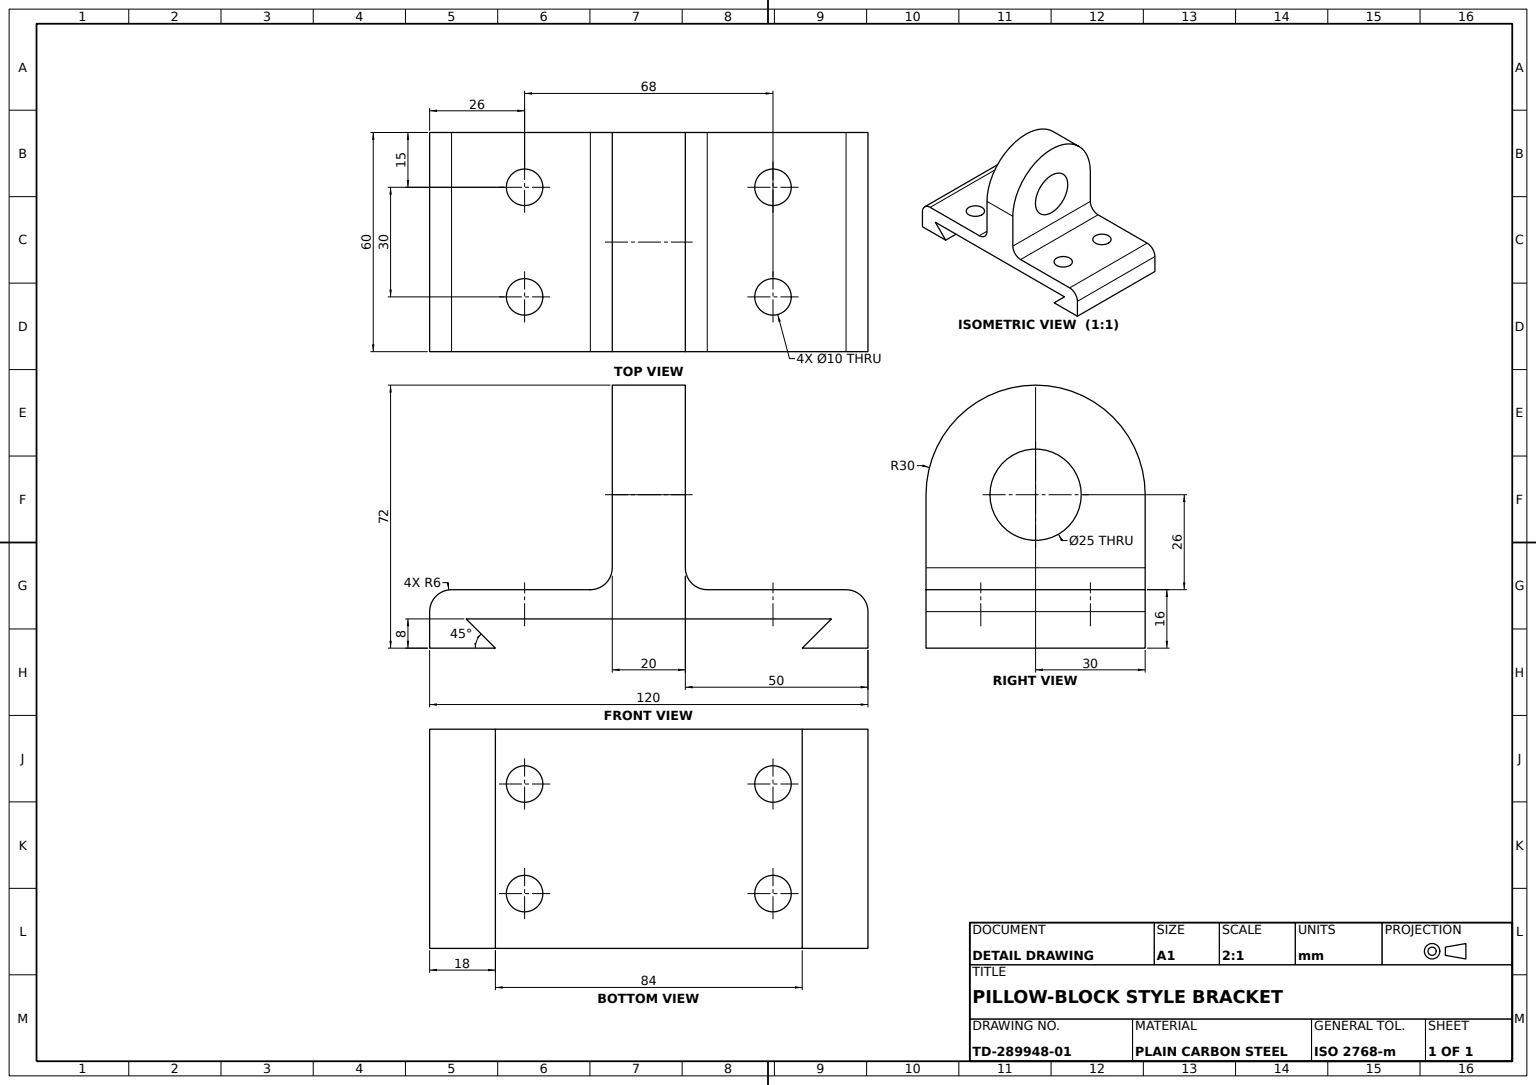
SolidWorks part; units mm, degrees
material "Plain Carbon Steel"
ref_plane "Front Plane" through (0, 0, 0) normal (0, 0, 1) x (1, 0, 0)
ref_plane "Top Plane" through (0, 0, 0) normal (0, 1, 0) x (1, 0, 0)
ref_plane "Right Plane" through (0, 0, 0) normal (1, 0, 0) x (0, 0, -1)
sketch "Base Plate Profile" plane through (0, 0, 0) normal (0, 0, 1) x (1, 0, 0)
  line L0 (0, 0) -> (50, 0)
  line L1 (50, 0) -> (42, -8)
  line L2 (42, -8) -> (60, -8)
  line L3 (60, -8) -> (60, 8)
  line L4 (60, 8) -> (-60, 8)
  line L5 (-60, 8) -> (-60, -8)
  line L6 (-60, -8) -> (-42, -8)
  line L7 (-42, -8) -> (-50, 0)
  line L8 (-50, 0) -> (0, 0)
  dimension "D1" = 16
  dimension "D2" = 18
  dimension "D3" = 120
  dimension "D4" = 18
  dimension "D5" = 45
  dimension "D6" = 45
  dimension "D7" = 16
  dimension "D8" = 60
  dimension "D9" = 10
extrude "Base Plate" add sketch "Base Plate Profile" against normal blind 60
sketch "Mounting Holes Sketch" plane through (0, 8, 0) normal (0, 1, 0) x (1, 0, 0)
  line L0 (60, 60) -> (-60, 60) construction
  circle A0 centre (34, 45) radius 5
  circle A1 centre (34, 15) radius 5
  circle A2 centre (-34, 45) radius 5
  circle A3 centre (-34, 15) radius 5
  dimension "D1" = 15
  dimension "D5" = 10
  dimension "D2" = 30
  dimension "D3" = 68
  dimension "D4" = 34
extrude "Mounting Holes" cut sketch "Mounting Holes Sketch" against normal blind 60
sketch "Eye Upright Profile" plane through (0, 0, 0) normal (1, 0, 0) x (0, 0, -1)
  line L0 (30, 8) -> (30, 34) construction
  line L1 (60, 8) -> (0, 8) construction
  line L2 (0, 8) -> (0, 34)
  line L3 (60, 8) -> (60, 34)
  line L4 (0, 8) -> (60, 8)
  arc A0 (60, 34) -> (0, 34) centre (30, 34) ccw
  circle A1 centre (30, 34) radius 12.5
  dimension "D2" = 60
  dimension "D3" = 25
  dimension "D1" = 26
extrude "Eye Upright" add sketch "Eye Upright Profile" along normal mid plane 20
fillet "Upright Root Fillet R6" radius 6 4 edges at (-60, 8, -30) (-10, 8, -30) (10, 8, -30) (60, 8, -30)
